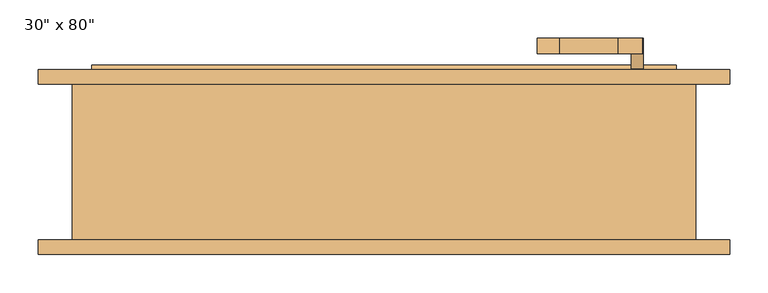
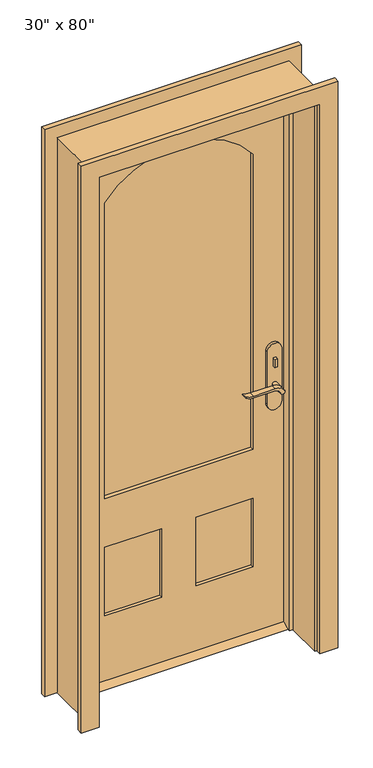
"""IFC4 building model written with IfcOpenShell, lengths in millimetres: door geometry."""

from ifc_helpers import new_model, si_unit, point, frame, frame_2d, origin, place, context, project, spatial, polyline, circle_curve, trimmed, segment, composite_curve, outline, extrude, faceted_brep, source, transform, mapped, element, save


def door_ad59dcae(model_context):
    return source(origin(), model_context, "Body", "SolidModel", [
        extrude(outline(polyline([(63.5, 12.7), (98.425, 12.7), (123.825, 0.0), (38.1, 0.0), (63.5, 12.7)])), frame((-381.0, 0.0, 0.0), z_axis=(1.0, 0.0, 0.0), x_axis=(0.0, 1.0, 0.0)), (0.0, 0.0, 1.0), 762.0),
        extrude(outline(polyline([(335.2, 43.5), (325.2, 43.5), (325.2, 53.5), (335.2, 53.5), (335.2, 43.5)])), frame((0.0, 0.0, 981.9), z_axis=(0.0, 0.0, 1.0), x_axis=(1.0, 0.0, 0.0)), (0.0, 0.0, 1.0), 30.0),
        extrude(outline(composite_curve([segment(trimmed(circle_curve(frame_2d((996.9, 330.2)), 8.0), [point((996.9, 322.2))], [point((996.9, 338.2))], False, "CARTESIAN"), True, "CONTINUOUS"), segment(trimmed(circle_curve(frame_2d((996.9, 330.2)), 8.0), [point((996.9, 338.2))], [point((996.9, 322.2))], False, "CARTESIAN"), True, "CONTINUOUS")], self_intersect=False)), frame((0.0, 108.425, 0.0), z_axis=(0.0, 1.0, 0.0), x_axis=(0.0, 0.0, 1.0)), (0.0, 0.0, 1.0), 10.0),
        extrude(outline(composite_curve([segment(trimmed(circle_curve(frame_2d((897.1555521, 306.5324871)), 37.2832219), [point((919.0523287, 336.7081363))], [point((934.4, 304.8325667))], False, "CARTESIAN"), True, "CONTINUOUS"), segment(polyline([(934.4, 304.8325667), (934.4, 228.5564091)]), True, "CONTINUOUS"), segment(trimmed(circle_curve(frame_2d((1017.6850638, 228.6227909)), 83.2850902), [point((934.4, 228.5564091))], [point((939.4, 200.2))], True, "CARTESIAN"), True, "CONTINUOUS"), segment(polyline([(939.4, 200.2), (936.6135558, 200.2)]), True, "CONTINUOUS"), segment(trimmed(circle_curve(frame_2d((986.6709207, 232.1396612)), 59.3791355), [point((936.6135558, 200.2))], [point((927.4, 228.5564091))], False, "CARTESIAN"), True, "CONTINUOUS"), segment(polyline([(927.4, 228.5564091), (927.4, 304.8138099)]), True, "CONTINUOUS"), segment(trimmed(circle_curve(frame_2d((909.2738613, 304.8138099)), 18.1261387), [point((927.4, 304.8138099))], [point((914.4, 322.2))], True, "CARTESIAN"), True, "CONTINUOUS"), segment(trimmed(circle_curve(frame_2d((914.4, 330.2)), 8.0), [point((914.4, 322.2))], [point((919.0523287, 336.7081363))], False, "CARTESIAN"), True, "CONTINUOUS")], self_intersect=False)), frame((0.0, 3.5, 0.0), z_axis=(0.0, 1.0, 0.0), x_axis=(0.0, 0.0, 1.0)), (0.0, 0.0, 1.0), 20.0),
        extrude(outline(composite_curve([segment(trimmed(circle_curve(frame_2d((914.4, 330.2)), 8.0), [point((914.3999903, 322.2))], [point((919.0523287, 336.7081363))], False, "CARTESIAN"), True, "CONTINUOUS"), segment(trimmed(circle_curve(frame_2d((897.1555521, 306.5324871)), 37.2832219), [point((919.0523287, 336.7081363))], [point((934.4, 304.8325667))], False, "CARTESIAN"), True, "CONTINUOUS"), segment(polyline([(934.4, 304.8325667), (934.4, 228.5564091)]), True, "CONTINUOUS"), segment(trimmed(circle_curve(frame_2d((1017.6850638, 228.6227909)), 83.2850902), [point((934.4, 228.5564091))], [point((939.4, 200.2))], True, "CARTESIAN"), True, "CONTINUOUS"), segment(polyline([(939.4, 200.2), (936.6135558, 200.2)]), True, "CONTINUOUS"), segment(trimmed(circle_curve(frame_2d((986.6709207, 232.1396612)), 59.3791355), [point((936.6135558, 200.2))], [point((927.4, 228.5564091))], False, "CARTESIAN"), True, "CONTINUOUS"), segment(polyline([(927.4, 228.5564091), (927.4, 304.8138122)]), True, "CONTINUOUS"), segment(trimmed(circle_curve(frame_2d((909.2738682, 304.8138122)), 18.1261318), [point((927.4, 304.8138122))], [point((914.3999903, 322.2))], True, "CARTESIAN"), True, "CONTINUOUS")], self_intersect=False)), frame((0.0, 138.425, 0.0), z_axis=(0.0, 1.0, 0.0), x_axis=(0.0, 0.0, 1.0)), (0.0, 0.0, 1.0), 20.0),
        extrude(outline(composite_curve([segment(trimmed(circle_curve(frame_2d((914.4, 330.2)), 8.0), [point((914.4, 322.2))], [point((914.4, 338.2))], False, "CARTESIAN"), True, "CONTINUOUS"), segment(trimmed(circle_curve(frame_2d((914.4, 330.2)), 8.0), [point((914.4, 338.2))], [point((914.4, 322.2))], False, "CARTESIAN"), True, "CONTINUOUS")], self_intersect=False)), frame((0.0, 23.5, 0.0), z_axis=(0.0, 1.0, 0.0), x_axis=(0.0, 0.0, 1.0)), (0.0, 0.0, 1.0), 30.0),
        extrude(outline(composite_curve([segment(trimmed(circle_curve(frame_2d((914.4, 330.2)), 8.0), [point((914.4, 322.2))], [point((914.4, 338.2))], False, "CARTESIAN"), True, "CONTINUOUS"), segment(trimmed(circle_curve(frame_2d((914.4, 330.2)), 8.0), [point((914.4, 338.2))], [point((914.4, 322.2))], False, "CARTESIAN"), True, "CONTINUOUS")], self_intersect=False)), frame((0.0, 108.425, 0.0), z_axis=(0.0, 1.0, 0.0), x_axis=(0.0, 0.0, 1.0)), (0.0, 0.0, 1.0), 30.0),
        extrude(outline(composite_curve([segment(polyline([(844.4, 355.2), (1039.4, 355.2)]), True, "CONTINUOUS"), segment(trimmed(circle_curve(frame_2d((1039.4, 330.2)), 25.0), [point((1039.4, 355.2))], [point((1039.4, 305.2))], False, "CARTESIAN"), True, "CONTINUOUS"), segment(polyline([(1039.4, 305.2), (844.4, 305.2)]), True, "CONTINUOUS"), segment(trimmed(circle_curve(frame_2d((844.4, 330.2)), 25.0), [point((844.4, 305.2))], [point((844.4, 355.2))], False, "CARTESIAN"), True, "CONTINUOUS")], self_intersect=False)), frame((0.0, 53.5, 0.0), z_axis=(0.0, 1.0, 0.0), x_axis=(0.0, 0.0, 1.0)), (0.0, 0.0, 1.0), 10.0),
        extrude(outline(composite_curve([segment(polyline([(844.4, 355.2), (1039.4, 355.2)]), True, "CONTINUOUS"), segment(trimmed(circle_curve(frame_2d((1039.4, 330.2)), 25.0), [point((1039.4, 355.2))], [point((1039.4, 305.2))], False, "CARTESIAN"), True, "CONTINUOUS"), segment(polyline([(1039.4, 305.2), (844.4, 305.2)]), True, "CONTINUOUS"), segment(trimmed(circle_curve(frame_2d((844.4, 330.2)), 25.0), [point((844.4, 305.2))], [point((844.4, 355.2))], False, "CARTESIAN"), True, "CONTINUOUS")], self_intersect=False)), frame((0.0, 98.425, 0.0), z_axis=(0.0, 1.0, 0.0), x_axis=(0.0, 0.0, 1.0)), (0.0, 0.0, 1.0), 10.0),
        extrude(outline(polyline([(2032.0, -381.0), (12.7, -381.0), (12.7, 381.0), (2032.0, 381.0), (2032.0, -381.0)]), holes=[composite_curve([segment(polyline([(688.975, -260.35), (1784.35, -260.35)]), True, "CONTINUOUS"), segment(trimmed(circle_curve(frame_2d((1580.99125, 0.0)), 330.35875), [point((1784.35, -260.35))], [point((1784.35, 260.35))], True, "CARTESIAN"), True, "CONTINUOUS"), segment(polyline([(1784.35, 260.35), (688.975, 260.35), (688.975, -260.35)]), True, "CONTINUOUS")], self_intersect=False), polyline([(508.0, -60.325), (254.0, -60.325), (254.0, -260.35), (508.0, -260.35), (508.0, -60.325)]), polyline([(508.0, 260.35), (254.0, 260.35), (254.0, 60.325), (508.0, 60.325), (508.0, 260.35)])]), frame((0.0, 63.5, 0.0), z_axis=(0.0, 1.0, 0.0), x_axis=(0.0, 0.0, 1.0)), (0.0, 0.0, 1.0), 34.925),
        faceted_brep([(406.4, 98.425, 0.0), (406.4, -104.775, 0.0), (381.0, -104.775, 0.0), (381.0, 28.575, 0.0), (368.3, 28.575, 0.0), (368.3, 63.5, 0.0), (381.0, 63.5, 0.0), (381.0, 98.425, 0.0), (406.4, 98.425, 2057.4), (406.4, -104.775, 2057.4), (-406.4, -104.775, 2057.4), (-406.4, -104.775, 0.0), (-381.0, -104.775, 0.0), (-381.0, -104.775, 2032.0), (381.0, -104.775, 2032.0), (381.0, 28.575, 2032.0), (-381.0, 28.575, 2032.0), (-381.0, 28.575, 0.0), (-368.3, 28.575, 0.0), (-368.3, 28.575, 2019.3), (368.3, 28.575, 2019.3), (368.3, 63.5, 2019.3), (-368.3, 63.5, 2019.3), (-368.3, 63.5, 0.0), (-381.0, 63.5, 0.0), (-381.0, 63.5, 2032.0), (381.0, 63.5, 2032.0), (381.0, 98.425, 2032.0), (-381.0, 98.425, 2032.0), (-381.0, 98.425, 0.0), (-406.4, 98.425, 0.0), (-406.4, 98.425, 2057.4)], [[[0, 1, 2, 3, 4, 5, 6, 7]], [[1, 0, 8, 9]], [[2, 1, 9, 10, 11, 12, 13, 14]], [[3, 2, 14, 15]], [[4, 3, 15, 16, 17, 18, 19, 20]], [[5, 4, 20, 21]], [[6, 5, 21, 22, 23, 24, 25, 26]], [[7, 6, 26, 27]], [[0, 7, 27, 28, 29, 30, 31, 8]], [[9, 8, 31, 10]], [[15, 14, 13, 16]], [[21, 20, 19, 22]], [[27, 26, 25, 28]], [[30, 29, 24, 23, 18, 17, 12, 11]], [[10, 31, 30, 11]], [[16, 13, 12, 17]], [[22, 19, 18, 23]], [[28, 25, 24, 29]]]),
        extrude(outline(polyline([(-60.325, 75.1416667), (-260.35, 75.1416667), (-260.35, 86.7833333), (-60.325, 86.7833333), (-60.325, 75.1416667)])), frame((0.0, 0.0, 254.0), z_axis=(0.0, 0.0, 1.0), x_axis=(1.0, 0.0, 0.0)), (0.0, 0.0, 1.0), 254.0),
        extrude(outline(polyline([(260.35, 75.1416667), (60.325, 75.1416667), (60.325, 86.7833333), (260.35, 86.7833333), (260.35, 75.1416667)])), frame((0.0, 0.0, 254.0), z_axis=(0.0, 0.0, 1.0), x_axis=(1.0, 0.0, 0.0)), (0.0, 0.0, 1.0), 254.0),
        extrude(outline(composite_curve([segment(polyline([(688.975, -260.35), (688.975, 260.35), (1784.35, 260.35)]), True, "CONTINUOUS"), segment(trimmed(circle_curve(frame_2d((1580.99125, 0.0)), 330.35875), [point((1784.35, 260.35))], [point((1784.35, -260.35))], False, "CARTESIAN"), True, "CONTINUOUS"), segment(polyline([(1784.35, -260.35), (688.975, -260.35)]), True, "CONTINUOUS")], self_intersect=False)), frame((0.0, 77.47, 0.0), z_axis=(0.0, 1.0, 0.0), x_axis=(0.0, 0.0, 1.0)), (0.0, 0.0, 1.0), 6.985),
        extrude(outline(polyline([(0.0, -450.85), (0.0, -387.35), (2038.35, -387.35), (2038.35, 387.35), (0.0, 387.35), (0.0, 450.85), (2101.85, 450.85), (2101.85, -450.85), (0.0, -450.85)])), frame((0.0, -123.825, 0.0), z_axis=(0.0, 1.0, 0.0), x_axis=(0.0, 0.0, 1.0)), (0.0, 0.0, 1.0), 19.05),
        extrude(outline(polyline([(0.0, -450.85), (0.0, -387.35), (2038.35, -387.35), (2038.35, 387.35), (0.0, 387.35), (0.0, 450.85), (2101.85, 450.85), (2101.85, -450.85), (0.0, -450.85)])), frame((0.0, 98.425, 0.0), z_axis=(0.0, 1.0, 0.0), x_axis=(0.0, 0.0, 1.0)), (0.0, 0.0, 1.0), 19.05),
    ])


if __name__ == "__main__":
    model = new_model("IFC4")
    model_context = context("Model", 3, world=origin())
    ifc_project = project(units=[si_unit("LENGTHUNIT", "METRE", prefix="MILLI")], contexts=[model_context])
    site = spatial("IfcSite", under=ifc_project)
    building = spatial("IfcBuilding", under=site)
    placement = place(None, origin())
    door_shape = door_ad59dcae(model_context)
    element("IfcDoor", 1, ObjectType="30\" x 80\"", at=placement, inside=building, context=model_context, shape_type="MappedRepresentation", body=[
        mapped(door_shape, transform((0.0, 0.0, 0.0), x_axis=(1.0, 0.0, 0.0), y_axis=(0.0, 1.0, 0.0), z_axis=(0.0, 0.0, 1.0))),
    ])
    save(model, "model.ifc")

# Revit data of these elements
# Type "30\" x 80\""
#   Type Mark = "8"
#   Assembly Code = "B2030100"
#   Analytic Construction = "French door, wood frame with single glass"
#   Threshold Offset [instance default] = 0' - 0 1/2"
#   Thickness = 0' - 1 3/8"
#   Thermal Resistance (R) = 1.0696 (h·ft²·°F)/BTU
#   Swing Angle [instance default] = 90.00°
#   Stiles = 0' - 4 3/4"
#   Rough Width = 2' - 8"
#   Rough Height = 6' - 9"
#   Radius = 1' - 1.00625"
#   Lock Rail = 0' - 7 1/8"
#   Height = 6' - 8"
#   Width = 2' - 6"
#   Heat Transfer Coefficient (U) = 0.9350 BTU/(h·ft²·°F)
#   Door Offset [instance default] = 0' - 0"
#   Bottom Rail = 0' - 9 1/2"
#   Threshold [instance default] = yes
#   Function = 1
#   Exterior Trim [instance default] = yes
#   Trim Material = Cherry
#   Threshold Material = Cherry
#   Panel Material = Cherry
#   Glazing = Glass
#   Frame Material = Cherry
#   Door Handle Material = Aluminum
#   Visual Light Transmittance = 0
#   Solar Heat Gain Coefficient = 0
#   Wall Closure = (empty or 0)
#   Construction Type = (empty or 0)
# Element 1 (IfcDoor, "30\" x 80\"")
#   Materials on its faces: "Cherry", "Aluminum", "Glass"
# Materials
#   "Cherry": class "Wood", colour RGB 226 177 128, transparency 0, Description = "Prunus Serotina", Cost = 0
#   "Glass": class "Glass", colour RGB 0 128 192, transparency 0.75, Description = "Soda Lime Glass", Cost = 0
#   "Aluminum": class "Metal", colour RGB 247 247 247, transparency 0, Description = "Aluminum 6061", Cost = 0
